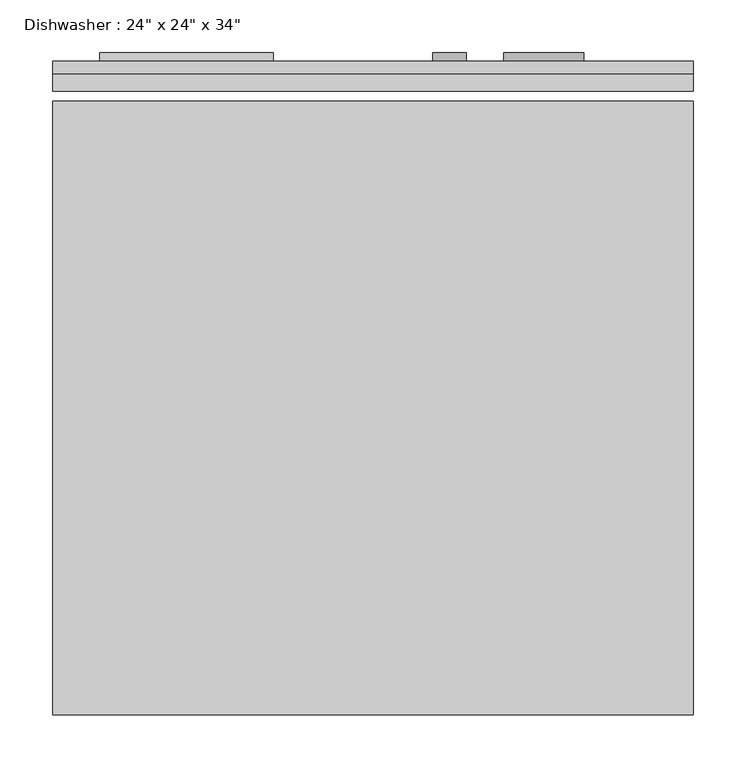
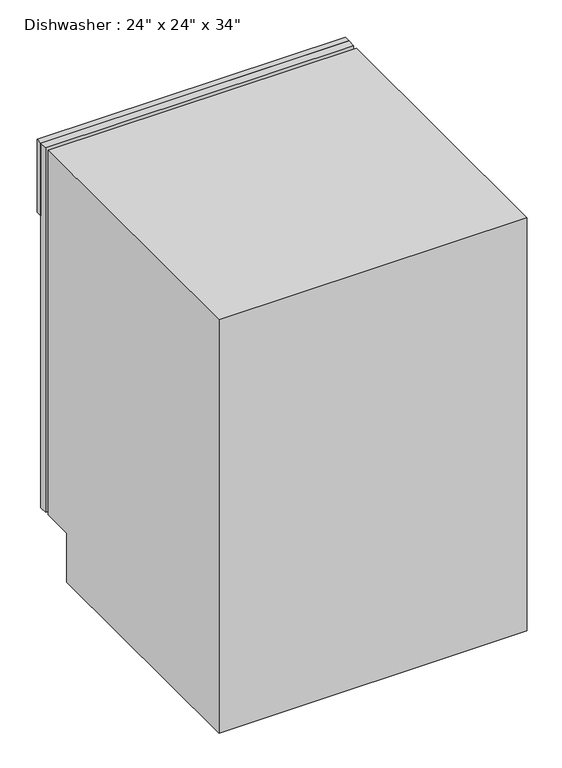
"""IFC4 building model written with IfcOpenShell, lengths in millimetres: proxy geometry."""

from ifc_helpers import new_model, si_unit, point, frame, frame_2d, origin, place, context, project, spatial, polyline, circle_curve, trimmed, segment, composite_curve, outline, extrude, source, transform, mapped, element, save


def proxy_3c49123c(model_context):
    return source(origin(), model_context, "Body", "SweptSolid", [
        extrude(outline(polyline([(687.1174685, 38.3504352), (687.1174685, 22.4754352), (77.5174685, 22.4754352), (77.5174685, 38.3504352), (687.1174685, 38.3504352)])), frame((0.0, 0.0, 101.6), z_axis=(0.0, 0.0, 1.0), x_axis=(1.0, 0.0, 0.0)), (0.0, 0.0, 1.0), 762.0),
        extrude(outline(polyline([(687.1174685, 38.3504352), (77.5174685, 38.3504352), (77.5174685, 51.0504352), (687.1174685, 51.0504352), (687.1174685, 38.3504352)])), frame((0.0, 0.0, 711.2), z_axis=(0.0, 0.0, 1.0), x_axis=(1.0, 0.0, 0.0)), (0.0, 0.0, 1.0), 152.4),
        extrude(outline(polyline([(-571.2495648, 0.0), (-571.2495648, 863.6), (12.9504352, 863.6), (12.9504352, 101.6), (-50.5495648, 101.6), (-50.5495648, 0.0), (-571.2495648, 0.0)])), frame((77.5174685, 0.0, 0.0), z_axis=(1.0, 0.0, 0.0), x_axis=(0.0, 1.0, 0.0)), (0.0, 0.0, 1.0), 609.6),
        extrude(outline(polyline([(287.6378068, 59.1863727), (287.6378068, 51.0504352), (122.5378068, 51.0504352), (122.5378068, 59.1863727), (287.6378068, 59.1863727)])), frame((0.0, 0.0, 780.0846419), z_axis=(0.0, 0.0, 1.0), x_axis=(1.0, 0.0, 0.0)), (0.0, 0.0, 1.0), 50.8),
        extrude(outline(composite_curve([segment(trimmed(circle_curve(frame_2d((780.0846419, 544.7247133)), 38.1), [point((780.0846419, 506.6247133))], [point((780.0846419, 582.8247133))], False, "CARTESIAN"), True, "CONTINUOUS"), segment(trimmed(circle_curve(frame_2d((780.0846419, 544.7247133)), 38.1), [point((780.0846419, 582.8247133))], [point((780.0846419, 506.6247133))], False, "CARTESIAN"), True, "CONTINUOUS")], self_intersect=False)), frame((0.0, 51.0504352, 0.0), z_axis=(0.0, 1.0, 0.0), x_axis=(0.0, 0.0, 1.0)), (0.0, 0.0, 1.0), 8.1359375),
        extrude(outline(composite_curve([segment(trimmed(circle_curve(frame_2d((780.0846419, 455.195318)), 15.875), [point((780.0846419, 439.320318))], [point((780.0846419, 471.070318))], False, "CARTESIAN"), True, "CONTINUOUS"), segment(trimmed(circle_curve(frame_2d((780.0846419, 455.195318)), 15.875), [point((780.0846419, 471.070318))], [point((780.0846419, 439.320318))], False, "CARTESIAN"), True, "CONTINUOUS")], self_intersect=False)), frame((0.0, 51.0504352, 0.0), z_axis=(0.0, 1.0, 0.0), x_axis=(0.0, 0.0, 1.0)), (0.0, 0.0, 1.0), 8.1359375),
    ])


if __name__ == "__main__":
    model = new_model("IFC4")
    model_context = context("Model", 3, world=origin())
    ifc_project = project(units=[si_unit("LENGTHUNIT", "METRE", prefix="MILLI")], contexts=[model_context])
    site = spatial("IfcSite", under=ifc_project)
    building = spatial("IfcBuilding", under=site)
    placement = place(None, origin())
    proxy_shape = proxy_3c49123c(model_context)
    element("IfcBuildingElementProxy", 1, Name="Dishwasher : 24\" x 24\" x 34\"", ObjectType="Dishwasher : 24\" x 24\" x 34\"", at=placement, inside=building, context=model_context, shape_type="MappedRepresentation", body=[
        mapped(proxy_shape, transform((0.0, 0.0, 0.0), x_axis=(1.0, 0.0, 0.0), y_axis=(0.0, 1.0, 0.0), z_axis=(0.0, 0.0, 1.0))),
    ])
    save(model, "model.ifc")

# Revit data of these elements
# Type "Dishwasher : 24\" x 24\" x 34\""
#   Label = "DW"
#   Assembly Code = "E1090400"
#   Depth = 2' - 0"
#   Height = 2' - 10"
#   Width = 2' - 0"
#   Dishwasher Material = Steel, Paint Finish, Ivory, Glossy
#   Panel Face Material = Plastic, Opaque Black
#   Default Elevation = 0
# Element 1 (IfcBuildingElementProxy, "Dishwasher : 24\" x 24\" x 34\"")
#   Materials on its faces: "Steel, Paint Finish, Ivory, Glossy", "Plastic, Opaque Black"
# Materials
#   "Steel, Paint Finish, Ivory, Glossy": class "Metal", colour RGB 247 247 239, transparency 0, Description = "Steel, paint finish, ivory, glossy", Cost = 0
#   "Plastic, Opaque Black": class "Plastic", colour RGB 0 0 0, transparency 0.7, Description = "Plastic, generic, opaque black", Cost = 0
